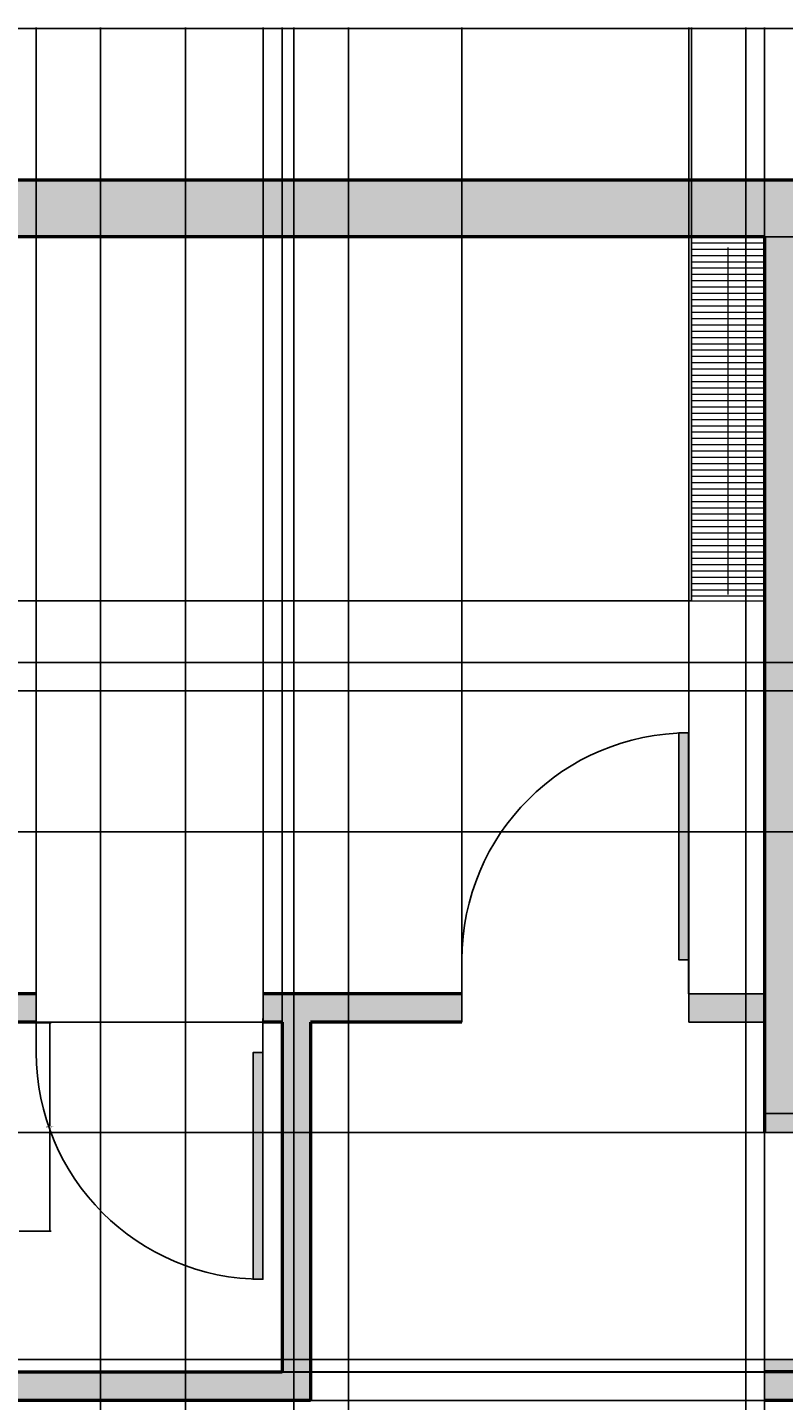
# Model space of a CAD drawing. Units: inches. Extents: x 1201 to 1754, y 247 to 775.
# Tile 8 of 10: x 1355 to 1475, y 557 to 775. Entities that reach past the tile are written whole.
import ezdxf

# ---------------------------------------------------------------- set-up
doc = ezdxf.new("R2010")
doc.units = ezdxf.units.IN
for name, color, linetype, lineweight in [('A-ANNO-DIMS', 2, 'Continuous', 18), ('A-DOOR', 4, 'Continuous', 25), ('A-FLOR-PANL', 8, 'Continuous', 18), ('A-FLOR-PANL-PATT', 8, 'Continuous', 13), ('A-WALL', 7, 'Continuous', 50), ('A-WALL-PATT', 9, 'Continuous', 13)]:
    doc.layers.add(name, color=color, linetype=linetype, lineweight=lineweight)
doc.layers.add('A-DOOR-PATT', color=29, linetype='Continuous', lineweight=13, true_color=0x4f342a)
doc.styles.get("Standard").update_dxf_attribs({"font": 'arial.ttf'})
doc.dimstyles.get("Standard").update_dxf_attribs({"dimtxt": 0.18, "dimasz": 0.18, "dimexe": 0.18, "dimexo": 0.0625, "dimgap": 0.09, "dimtad": 0, "dimtih": 1, "dimtoh": 1, "dimdec": 4, "dimzin": 0, "dimdsep": 46, "dimtxsty": 'Standard', "dimcen": 0.09, "dimadec": 0, "dimazin": 0, "dimtfac": 1, "dimtdec": 4, "dimtofl": 0, "dimtmove": 0, "dimatfit": 3, "dimfxl": 1, "dimtolj": 1, "dimtzin": 0, "dimarcsym": 0})

# ---------------------------------------------------------------- blocks, each defined once
blk = doc.blocks.new('*U2')
for p, q in [((0, 0), (0, -6)), ((-40, 0), (-40, -6))]:
    blk.add_line(p, q)
blk.add_lwpolyline([(0, 0), (0, 40), (-1.75, 40), (-1.75, 0)], close=True)
blk.add_arc((0, 0), 40, 90, 180)
blk = doc.blocks.new('*U3')
for p, q in [((0, 0), (0, -6)), ((40, 0), (40, -6))]:
    blk.add_line(p, q)
blk.add_lwpolyline([(0, 0), (0, 40), (1.75, 40), (1.75, 0)], close=True)
blk.add_arc((0, 0), 40, 0, 90)
blk = doc.blocks.new('*D27')
at = {"layer": 'A-ANNO-DIMS', "color": 0, "lineweight": -2, "transparency": 16777216}
for p, q in [((1353.29, 617.33), (1358.37, 617.33)), ((1358.19, 617.15), (1358.19, 600.99)), ((1358.19, 584.47), (1358.19, 600.63)), ((1353.29, 584.29), (1358.37, 584.29))]:
    blk.add_line(p, q, dxfattribs=at)
at = {"layer": 'A-ANNO-DIMS', "color": 0, "transparency": 16777216}
for points in [[(1358.16, 617.15), (1358.22, 617.15), (1358.19, 617.33)], [(1358.16, 584.47), (1358.22, 584.47), (1358.19, 584.29)]]:
    blk.add_solid(points, dxfattribs=at)
at = {"layer": 'Defpoints', "color": 0, "transparency": 16777216}
for p in [(1353.23, 617.33), (1358.19, 617.33), (1353.23, 584.29)]:
    blk.add_point(p, dxfattribs=at)
at = {"layer": 'A-ANNO-DIMS', "color": 0, "transparency": 16777216, "insert": (1358.19, 600.81), "char_height": 0.18, "attachment_point": 5}
blk.add_mtext('\\A1;WC 33 TYP.', dxfattribs=at)
blk = doc.blocks.new('*D45')
at = {"layer": 'A-ANNO-DIMS', "color": 0, "lineweight": -2, "transparency": 16777216}
for p, q in [((1246.52, 751), (1246.52, 775.14)), ((1726.52, 751), (1726.52, 775.14)), ((1246.7, 774.96), (1486.23, 774.96)), ((1726.34, 774.96), (1486.81, 774.96))]:
    blk.add_line(p, q, dxfattribs=at)
at = {"layer": 'A-ANNO-DIMS', "color": 0, "transparency": 16777216}
for points in [[(1246.7, 774.99), (1246.7, 774.93), (1246.52, 774.96)], [(1726.34, 774.99), (1726.34, 774.93), (1726.52, 774.96)]]:
    blk.add_solid(points, dxfattribs=at)
at = {"layer": 'Defpoints', "color": 0, "transparency": 16777216}
for p in [(1726.52, 774.96), (1246.52, 750.94), (1726.52, 750.94)]:
    blk.add_point(p, dxfattribs=at)
at = {"layer": 'A-ANNO-DIMS', "color": 0, "transparency": 16777216, "insert": (1486.52, 774.96), "char_height": 0.18, "attachment_point": 5}
blk.add_mtext('\\A1;480', dxfattribs=at)
blk = doc.blocks.new('*D47')
at = {"layer": 'A-ANNO-DIMS', "color": 0, "lineweight": -2, "transparency": 16777216}
for p, q in [((1255.52, 742), (1255.52, 775.14)), ((1471.52, 742), (1471.52, 775.14)), ((1255.7, 774.96), (1363.23, 774.96)), ((1471.34, 774.96), (1363.81, 774.96))]:
    blk.add_line(p, q, dxfattribs=at)
at = {"layer": 'A-ANNO-DIMS', "color": 0, "transparency": 16777216}
for points in [[(1255.7, 774.99), (1255.7, 774.93), (1255.52, 774.96)], [(1471.34, 774.99), (1471.34, 774.93), (1471.52, 774.96)]]:
    blk.add_solid(points, dxfattribs=at)
at = {"layer": 'Defpoints', "color": 0, "transparency": 16777216}
for p in [(1471.52, 774.96), (1255.52, 741.94), (1471.52, 741.94)]:
    blk.add_point(p, dxfattribs=at)
at = {"layer": 'A-ANNO-DIMS', "color": 0, "transparency": 16777216, "insert": (1363.52, 774.96), "char_height": 0.18, "attachment_point": 5}
blk.add_mtext('\\A1;216', dxfattribs=at)
blk = doc.blocks.new('*D49')
at = {"layer": 'A-ANNO-DIMS', "color": 0, "lineweight": -2, "transparency": 16777216}
for p, q in [((1394.96, 617.44), (1222.33, 617.44)), ((1222.51, 617.26), (1222.51, 589.87)), ((1222.51, 562.12), (1222.51, 589.51)), ((1394.96, 561.94), (1222.33, 561.94))]:
    blk.add_line(p, q, dxfattribs=at)
at = {"layer": 'A-ANNO-DIMS', "color": 0, "transparency": 16777216}
for points in [[(1222.48, 617.26), (1222.54, 617.26), (1222.51, 617.44)], [(1222.48, 562.12), (1222.54, 562.12), (1222.51, 561.94)]]:
    blk.add_solid(points, dxfattribs=at)
at = {"layer": 'Defpoints', "color": 0, "transparency": 16777216}
for p in [(1222.51, 617.44), (1395.02, 617.44), (1395.02, 561.94)]:
    blk.add_point(p, dxfattribs=at)
at = {"layer": 'A-ANNO-DIMS', "color": 0, "transparency": 16777216, "insert": (1222.51, 589.69), "char_height": 0.18, "attachment_point": 5}
blk.add_mtext('\\A1;55.5', dxfattribs=at)
blk = doc.blocks.new('*D52')
at = {"layer": 'A-ANNO-DIMS', "color": 0, "lineweight": -2, "transparency": 16777216}
for p, q in [((1477.46, 669.94), (1222.33, 669.94)), ((1222.51, 669.76), (1222.51, 616.12)), ((1222.51, 562.12), (1222.51, 615.76)), ((1477.46, 561.94), (1222.33, 561.94))]:
    blk.add_line(p, q, dxfattribs=at)
at = {"layer": 'A-ANNO-DIMS', "color": 0, "transparency": 16777216}
for points in [[(1222.48, 669.76), (1222.54, 669.76), (1222.51, 669.94)], [(1222.48, 562.12), (1222.54, 562.12), (1222.51, 561.94)]]:
    blk.add_solid(points, dxfattribs=at)
at = {"layer": 'Defpoints', "color": 0, "transparency": 16777216}
for p in [(1222.51, 669.94), (1477.52, 669.94), (1477.52, 561.94)]:
    blk.add_point(p, dxfattribs=at)
at = {"layer": 'A-ANNO-DIMS', "color": 0, "transparency": 16777216, "insert": (1222.51, 615.94), "char_height": 0.18, "attachment_point": 5}
blk.add_mtext('\\A1;108', dxfattribs=at)
blk = doc.blocks.new('*D53')
at = {"layer": 'A-ANNO-DIMS', "color": 0, "lineweight": -2, "transparency": 16777216}
for p, q in [((1717.46, 741.94), (1222.33, 741.94)), ((1222.51, 741.76), (1222.51, 708.37)), ((1222.51, 674.62), (1222.51, 708.01)), ((1657.46, 674.44), (1222.33, 674.44))]:
    blk.add_line(p, q, dxfattribs=at)
at = {"layer": 'A-ANNO-DIMS', "color": 0, "transparency": 16777216}
for points in [[(1222.48, 741.76), (1222.54, 741.76), (1222.51, 741.94)], [(1222.48, 674.62), (1222.54, 674.62), (1222.51, 674.44)]]:
    blk.add_solid(points, dxfattribs=at)
at = {"layer": 'Defpoints', "color": 0, "transparency": 16777216}
for p in [(1222.51, 741.94), (1717.52, 741.94), (1657.52, 674.44)]:
    blk.add_point(p, dxfattribs=at)
at = {"layer": 'A-ANNO-DIMS', "color": 0, "transparency": 16777216, "insert": (1222.51, 708.19), "char_height": 0.18, "attachment_point": 5}
blk.add_mtext('\\A1;67.5', dxfattribs=at)
blk = doc.blocks.new('*D54')
at = {"layer": 'A-ANNO-DIMS', "color": 0, "lineweight": -2, "transparency": 16777216}
for p, q in [((1255.52, 562), (1255.52, 775.14)), ((1395.02, 562), (1395.02, 775.14)), ((1255.7, 774.96), (1324.88, 774.96)), ((1394.84, 774.96), (1325.66, 774.96))]:
    blk.add_line(p, q, dxfattribs=at)
at = {"layer": 'A-ANNO-DIMS', "color": 0, "transparency": 16777216}
for points in [[(1255.7, 774.99), (1255.7, 774.93), (1255.52, 774.96)], [(1394.84, 774.99), (1394.84, 774.93), (1395.02, 774.96)]]:
    blk.add_solid(points, dxfattribs=at)
at = {"layer": 'Defpoints', "color": 0, "transparency": 16777216}
for p in [(1395.02, 774.96), (1255.52, 561.94), (1395.02, 561.94)]:
    blk.add_point(p, dxfattribs=at)
at = {"layer": 'A-ANNO-DIMS', "color": 0, "transparency": 16777216, "insert": (1325.27, 774.96), "char_height": 0.18, "attachment_point": 5}
blk.add_mtext('\\A1;139.5', dxfattribs=at)
blk = doc.blocks.new('*D58')
at = {"layer": 'A-ANNO-DIMS', "color": 0, "lineweight": -2, "transparency": 16777216}
for p, q in [((1405.52, 418), (1405.52, 775.14)), ((1468.52, 418), (1468.52, 775.14)), ((1405.7, 774.96), (1436.8, 774.96)), ((1468.34, 774.96), (1437.24, 774.96))]:
    blk.add_line(p, q, dxfattribs=at)
at = {"layer": 'A-ANNO-DIMS', "color": 0, "transparency": 16777216}
for points in [[(1405.7, 774.99), (1405.7, 774.93), (1405.52, 774.96)], [(1468.34, 774.99), (1468.34, 774.93), (1468.52, 774.96)]]:
    blk.add_solid(points, dxfattribs=at)
at = {"layer": 'Defpoints', "color": 0, "transparency": 16777216}
for p in [(1468.52, 774.96), (1405.52, 417.94), (1468.52, 417.94)]:
    blk.add_point(p, dxfattribs=at)
at = {"layer": 'A-ANNO-DIMS', "color": 0, "transparency": 16777216, "insert": (1437.02, 774.96), "char_height": 0.18, "attachment_point": 5}
blk.add_mtext('\\A1;63', dxfattribs=at)
blk = doc.blocks.new('*D59')
at = {"layer": 'A-ANNO-DIMS', "color": 0, "lineweight": -2, "transparency": 16777216}
for p, q in [((1255.52, 418), (1255.52, 775.14)), ((1405.52, 418), (1405.52, 775.14)), ((1255.7, 774.96), (1330.24, 774.96)), ((1405.34, 774.96), (1330.8, 774.96))]:
    blk.add_line(p, q, dxfattribs=at)
at = {"layer": 'A-ANNO-DIMS', "color": 0, "transparency": 16777216}
for points in [[(1255.7, 774.99), (1255.7, 774.93), (1255.52, 774.96)], [(1405.34, 774.99), (1405.34, 774.93), (1405.52, 774.96)]]:
    blk.add_solid(points, dxfattribs=at)
at = {"layer": 'Defpoints', "color": 0, "transparency": 16777216}
for p in [(1405.52, 774.96), (1255.52, 417.94), (1405.52, 417.94)]:
    blk.add_point(p, dxfattribs=at)
at = {"layer": 'A-ANNO-DIMS', "color": 0, "transparency": 16777216, "insert": (1330.52, 774.96), "char_height": 0.18, "attachment_point": 5}
blk.add_mtext('\\A1;150', dxfattribs=at)
blk = doc.blocks.new('*D61')
at = {"layer": 'A-ANNO-DIMS', "color": 0, "lineweight": -2, "transparency": 16777216}
for p, q in [((1423.52, 622), (1423.52, 775.14)), ((1459.52, 622), (1459.52, 775.14)), ((1423.7, 774.96), (1441.3, 774.96)), ((1459.34, 774.96), (1441.74, 774.96))]:
    blk.add_line(p, q, dxfattribs=at)
at = {"layer": 'A-ANNO-DIMS', "color": 0, "transparency": 16777216}
for points in [[(1423.7, 774.99), (1423.7, 774.93), (1423.52, 774.96)], [(1459.34, 774.99), (1459.34, 774.93), (1459.52, 774.96)]]:
    blk.add_solid(points, dxfattribs=at)
at = {"layer": 'Defpoints', "color": 0, "transparency": 16777216}
for p in [(1459.52, 774.96), (1423.52, 621.94), (1459.52, 621.94)]:
    blk.add_point(p, dxfattribs=at)
at = {"layer": 'A-ANNO-DIMS', "color": 0, "transparency": 16777216, "insert": (1441.52, 774.96), "char_height": 0.18, "attachment_point": 5}
blk.add_mtext('\\A1;36', dxfattribs=at)
blk = doc.blocks.new('*D62')
at = {"layer": 'A-ANNO-DIMS', "color": 0, "lineweight": -2, "transparency": 16777216}
for p, q in [((1459.52, 622), (1459.52, 775.14)), ((1471.52, 622), (1471.52, 775.14)), ((1459.7, 774.96), (1465.31, 774.96)), ((1471.34, 774.96), (1465.73, 774.96))]:
    blk.add_line(p, q, dxfattribs=at)
at = {"layer": 'A-ANNO-DIMS', "color": 0, "transparency": 16777216}
for points in [[(1459.7, 774.99), (1459.7, 774.93), (1459.52, 774.96)], [(1471.34, 774.99), (1471.34, 774.93), (1471.52, 774.96)]]:
    blk.add_solid(points, dxfattribs=at)
at = {"layer": 'Defpoints', "color": 0, "transparency": 16777216}
for p in [(1471.52, 774.96), (1459.52, 621.94), (1471.52, 621.94)]:
    blk.add_point(p, dxfattribs=at)
at = {"layer": 'A-ANNO-DIMS', "color": 0, "transparency": 16777216, "insert": (1465.52, 774.96), "char_height": 0.18, "attachment_point": 5}
blk.add_mtext('\\A1;12', dxfattribs=at)
blk = doc.blocks.new('*D63')
at = {"layer": 'A-ANNO-DIMS', "color": 0, "lineweight": -2, "transparency": 16777216}
for p, q in [((1356.02, 622), (1356.02, 775.14)), ((1392.02, 622), (1392.02, 775.14)), ((1356.2, 774.96), (1373.8, 774.96)), ((1391.84, 774.96), (1374.24, 774.96))]:
    blk.add_line(p, q, dxfattribs=at)
at = {"layer": 'A-ANNO-DIMS', "color": 0, "transparency": 16777216}
for points in [[(1356.2, 774.99), (1356.2, 774.93), (1356.02, 774.96)], [(1391.84, 774.99), (1391.84, 774.93), (1392.02, 774.96)]]:
    blk.add_solid(points, dxfattribs=at)
at = {"layer": 'Defpoints', "color": 0, "transparency": 16777216}
for p in [(1392.02, 774.96), (1356.02, 621.94), (1392.02, 621.94)]:
    blk.add_point(p, dxfattribs=at)
at = {"layer": 'A-ANNO-DIMS', "color": 0, "transparency": 16777216, "insert": (1374.02, 774.96), "char_height": 0.18, "attachment_point": 5}
blk.add_mtext('\\A1;36', dxfattribs=at)
blk = doc.blocks.new('*D64')
at = {"layer": 'A-ANNO-DIMS', "color": 0, "lineweight": -2, "transparency": 16777216}
for p, q in [((1392.02, 622), (1392.02, 775.14)), ((1423.52, 622), (1423.52, 775.14)), ((1392.2, 774.96), (1407.45, 774.96)), ((1423.34, 774.96), (1408.1, 774.96))]:
    blk.add_line(p, q, dxfattribs=at)
at = {"layer": 'A-ANNO-DIMS', "color": 0, "transparency": 16777216}
for points in [[(1392.2, 774.99), (1392.2, 774.93), (1392.02, 774.96)], [(1423.34, 774.99), (1423.34, 774.93), (1423.52, 774.96)]]:
    blk.add_solid(points, dxfattribs=at)
at = {"layer": 'Defpoints', "color": 0, "transparency": 16777216}
for p in [(1423.52, 774.96), (1392.02, 621.94), (1423.52, 621.94)]:
    blk.add_point(p, dxfattribs=at)
at = {"layer": 'A-ANNO-DIMS', "color": 0, "transparency": 16777216, "insert": (1407.77, 774.96), "char_height": 0.18, "attachment_point": 5}
blk.add_mtext('\\A1;31.5', dxfattribs=at)
blk = doc.blocks.new('*D65')
at = {"layer": 'A-ANNO-DIMS', "color": 0, "lineweight": -2, "transparency": 16777216}
for p, q in [((1471.46, 599.94), (1222.33, 599.94)), ((1222.51, 599.76), (1222.51, 582.12)), ((1222.51, 564.12), (1222.51, 581.76)), ((1471.46, 563.94), (1222.33, 563.94))]:
    blk.add_line(p, q, dxfattribs=at)
at = {"layer": 'A-ANNO-DIMS', "color": 0, "transparency": 16777216}
for points in [[(1222.48, 599.76), (1222.54, 599.76), (1222.51, 599.94)], [(1222.48, 564.12), (1222.54, 564.12), (1222.51, 563.94)]]:
    blk.add_solid(points, dxfattribs=at)
at = {"layer": 'Defpoints', "color": 0, "transparency": 16777216}
for p in [(1222.51, 599.94), (1471.52, 599.94), (1471.52, 563.94)]:
    blk.add_point(p, dxfattribs=at)
at = {"layer": 'A-ANNO-DIMS', "color": 0, "transparency": 16777216, "insert": (1222.51, 581.94), "char_height": 0.18, "attachment_point": 5}
blk.add_mtext('\\A1;36', dxfattribs=at)
blk = doc.blocks.new('*D76')
at = {"layer": 'A-ANNO-DIMS', "color": 0, "lineweight": -2, "transparency": 16777216}
for p, q in [((1717.46, 669.94), (1222.33, 669.94)), ((1222.51, 669.76), (1222.51, 658.95)), ((1222.51, 647.78), (1222.51, 658.59)), ((1717.46, 647.6), (1222.33, 647.6))]:
    blk.add_line(p, q, dxfattribs=at)
at = {"layer": 'A-ANNO-DIMS', "color": 0, "transparency": 16777216}
for points in [[(1222.48, 669.76), (1222.54, 669.76), (1222.51, 669.94)], [(1222.48, 647.78), (1222.54, 647.78), (1222.51, 647.6)]]:
    blk.add_solid(points, dxfattribs=at)
at = {"layer": 'Defpoints', "color": 0, "transparency": 16777216}
for p in [(1222.51, 669.94), (1717.52, 669.94), (1717.52, 647.6)]:
    blk.add_point(p, dxfattribs=at)
at = {"layer": 'A-ANNO-DIMS', "color": 0, "transparency": 16777216, "insert": (1222.51, 658.77), "char_height": 0.18, "attachment_point": 5}
blk.add_mtext('\\A1;22.34', dxfattribs=at)
blk = doc.blocks.new('*D83')
at = {"layer": 'A-ANNO-DIMS', "color": 0, "lineweight": -2, "transparency": 16777216}
for p, q in [((1471.46, 561.97), (1222.33, 561.97)), ((1222.51, 561.79), (1222.51, 559.89)), ((1222.51, 557.62), (1222.51, 559.52)), ((1471.46, 557.44), (1222.33, 557.44))]:
    blk.add_line(p, q, dxfattribs=at)
at = {"layer": 'A-ANNO-DIMS', "color": 0, "transparency": 16777216}
for points in [[(1222.48, 561.79), (1222.54, 561.79), (1222.51, 561.97)], [(1222.48, 557.62), (1222.54, 557.62), (1222.51, 557.44)]]:
    blk.add_solid(points, dxfattribs=at)
at = {"layer": 'Defpoints', "color": 0, "transparency": 16777216}
for p in [(1222.51, 561.97), (1471.52, 561.97), (1471.52, 557.44)]:
    blk.add_point(p, dxfattribs=at)
at = {"layer": 'A-ANNO-DIMS', "color": 0, "transparency": 16777216, "insert": (1222.51, 559.71), "char_height": 0.18, "attachment_point": 5}
blk.add_mtext('\\A1;4.528', dxfattribs=at)
blk = doc.blocks.new('*D84')
at = {"layer": 'A-ANNO-DIMS', "color": 0, "lineweight": -2, "transparency": 16777216}
for p, q in [((1471.52, 600), (1471.52, 775.14)), ((1477.52, 600), (1477.52, 775.14)), ((1471.7, 774.96), (1474.37, 774.96)), ((1477.34, 774.96), (1474.67, 774.96))]:
    blk.add_line(p, q, dxfattribs=at)
at = {"layer": 'A-ANNO-DIMS', "color": 0, "transparency": 16777216}
for points in [[(1471.7, 774.99), (1471.7, 774.93), (1471.52, 774.96)], [(1477.34, 774.99), (1477.34, 774.93), (1477.52, 774.96)]]:
    blk.add_solid(points, dxfattribs=at)
at = {"layer": 'Defpoints', "color": 0, "transparency": 16777216}
for p in [(1477.52, 774.96), (1471.52, 599.94), (1477.52, 599.94)]:
    blk.add_point(p, dxfattribs=at)
at = {"layer": 'A-ANNO-DIMS', "color": 0, "transparency": 16777216, "insert": (1474.52, 774.96), "char_height": 0.18, "attachment_point": 5}
blk.add_mtext('\\A1;6', dxfattribs=at)
blk = doc.blocks.new('*D87')
at = {"layer": 'A-ANNO-DIMS', "color": 0, "lineweight": -2, "transparency": 16777216}
for p, q in [((1459.84, 741.94), (1222.33, 741.94)), ((1222.51, 741.76), (1222.51, 713.27)), ((1222.51, 684.41), (1222.51, 712.91)), ((1459.84, 684.23), (1222.33, 684.23))]:
    blk.add_line(p, q, dxfattribs=at)
at = {"layer": 'A-ANNO-DIMS', "color": 0, "transparency": 16777216}
for points in [[(1222.48, 741.76), (1222.54, 741.76), (1222.51, 741.94)], [(1222.48, 684.41), (1222.54, 684.41), (1222.51, 684.23)]]:
    blk.add_solid(points, dxfattribs=at)
at = {"layer": 'Defpoints', "color": 0, "transparency": 16777216}
for p in [(1222.51, 741.94), (1459.9, 741.94), (1459.9, 684.23)]:
    blk.add_point(p, dxfattribs=at)
at = {"layer": 'A-ANNO-DIMS', "color": 0, "transparency": 16777216, "insert": (1222.51, 713.09), "char_height": 0.18, "attachment_point": 5}
blk.add_mtext('\\A1;57.71', dxfattribs=at)
blk = doc.blocks.new('*D88')
at = {"layer": 'A-ANNO-DIMS', "color": 0, "lineweight": -2, "transparency": 16777216}
for p, q in [((1459.9, 684.3), (1459.9, 775.14)), ((1471.52, 684.3), (1471.52, 775.14)), ((1460.08, 774.96), (1465.25, 774.96)), ((1471.34, 774.96), (1466.16, 774.96))]:
    blk.add_line(p, q, dxfattribs=at)
at = {"layer": 'A-ANNO-DIMS', "color": 0, "transparency": 16777216}
for points in [[(1460.08, 774.99), (1460.08, 774.93), (1459.9, 774.96)], [(1471.34, 774.99), (1471.34, 774.93), (1471.52, 774.96)]]:
    blk.add_solid(points, dxfattribs=at)
at = {"layer": 'Defpoints', "color": 0, "transparency": 16777216}
for p in [(1471.52, 774.96), (1459.9, 684.23), (1471.52, 684.23)]:
    blk.add_point(p, dxfattribs=at)
at = {"layer": 'A-ANNO-DIMS', "color": 0, "transparency": 16777216, "insert": (1465.71, 774.96), "char_height": 0.18, "attachment_point": 5}
blk.add_mtext('\\A1;11.623', dxfattribs=at)
blk = doc.blocks.new('*D89')
at = {"layer": 'A-ANNO-DIMS', "color": 0, "lineweight": -2, "transparency": 16777216}
for p, q in [((1396.89, 281.58), (1396.89, 775.14)), ((1471.52, 280), (1471.52, 775.14)), ((1397.07, 774.96), (1433.81, 774.96)), ((1471.34, 774.96), (1434.6, 774.96))]:
    blk.add_line(p, q, dxfattribs=at)
at = {"layer": 'A-ANNO-DIMS', "color": 0, "transparency": 16777216}
for points in [[(1397.07, 774.99), (1397.07, 774.93), (1396.89, 774.96)], [(1471.34, 774.99), (1471.34, 774.93), (1471.52, 774.96)]]:
    blk.add_solid(points, dxfattribs=at)
at = {"layer": 'Defpoints', "color": 0, "transparency": 16777216}
for p in [(1471.52, 774.96), (1396.89, 281.52), (1471.52, 279.94)]:
    blk.add_point(p, dxfattribs=at)
at = {"layer": 'A-ANNO-DIMS', "color": 0, "transparency": 16777216, "insert": (1434.21, 774.96), "char_height": 0.18, "attachment_point": 5}
blk.add_mtext('\\A1;74.63', dxfattribs=at)
blk = doc.blocks.new('*D98')
at = {"layer": 'A-ANNO-DIMS', "color": 0, "lineweight": -2, "transparency": 16777216}
for p, q in [((1366.21, 509.65), (1366.21, 775.14)), ((1379.71, 519.97), (1379.71, 775.14)), ((1366.39, 774.96), (1372.5, 774.96)), ((1379.53, 774.96), (1373.41, 774.96))]:
    blk.add_line(p, q, dxfattribs=at)
at = {"layer": 'A-ANNO-DIMS', "color": 0, "transparency": 16777216}
for points in [[(1366.39, 774.99), (1366.39, 774.93), (1366.21, 774.96)], [(1379.53, 774.99), (1379.53, 774.93), (1379.71, 774.96)]]:
    blk.add_solid(points, dxfattribs=at)
at = {"layer": 'Defpoints', "color": 0, "transparency": 16777216}
for p in [(1379.71, 774.96), (1379.71, 519.9), (1366.21, 509.58)]:
    blk.add_point(p, dxfattribs=at)
at = {"layer": 'A-ANNO-DIMS', "color": 0, "transparency": 16777216, "insert": (1372.96, 774.96), "char_height": 0.18, "attachment_point": 5}
blk.add_mtext('\\A1;13.494', dxfattribs=at)

msp = doc.modelspace()

# ---------------------------------------------------------------- hatches: boundary and pattern name
at = {"layer": 'A-DOOR-PATT'}
h = msp.add_hatch(color=256, dxfattribs=at)
h.dxf.hatch_style = 1
h.paths.add_polyline_path([(1391.9756, 612.6194), (1390.4026, 612.6194), (1390.4026, 576.699, 0.01094143), (1391.9756, 576.6646)])
h.paths.add_polyline_path([(1471.5208, 621.9415), (1459.5208, 621.9415), (1459.5208, 617.4415), (1471.5208, 617.4415)])
h.paths.add_polyline_path([(1459.4756, 663.2896, 0.01094143), (1457.9026, 663.2551), (1457.9026, 627.3347), (1459.4756, 627.3347)])
h.paths.add_polyline_path([(1477.5208, 602.9415), (1471.5208, 602.9415), (1471.5208, 599.9415), (1477.5208, 599.9415)])
h.paths.add_polyline_path([(1518.8344, 565.5145), (1482.914, 565.5145), (1482.914, 563.9415), (1518.8689, 563.9415, 0.01094143)])
h.paths.add_polyline_path([(1477.5208, 563.9415), (1471.5208, 563.9415), (1471.5208, 561.9692), (1477.5208, 561.9692)])
h.paths.add_polyline_path([(1621.5208, 674.4415), (1618.5208, 674.4415), (1618.5208, 669.9415), (1621.5208, 669.9415)])
h.paths.add_polyline_path([(1660.5208, 674.4415), (1657.5208, 674.4415), (1657.5208, 669.9415), (1660.5208, 669.9415)])
h.paths.add_polyline_path([(1657.509, 715.7896, 0.01094143), (1655.936, 715.7551), (1655.936, 679.8347), (1657.509, 679.8347)])
h.paths.add_polyline_path([(1566.0208, 279.9415), (1563.0208, 279.9415), (1563.0208, 270.9415), (1566.0208, 270.9415)])
h.paths.add_polyline_path([(1567.6389, 321.2551, 0.01094143), (1566.0659, 321.2896), (1566.0659, 285.3347), (1567.6389, 285.3347)])
h.paths.add_polyline_path([(1603.0208, 279.9415), (1602.0208, 279.9415), (1602.0208, 270.9415), (1603.0208, 270.9415)])
h.paths.add_polyline_path([(1641.0208, 279.9415), (1638.0208, 279.9415), (1638.0208, 270.9415), (1641.0208, 270.9415)])
h.paths.add_polyline_path([(1638.0208, 320.3922, 0.01094143), (1636.4477, 320.3578), (1636.4477, 284.4374), (1638.0208, 284.4374)])
at = {"layer": 'A-FLOR-PANL-PATT'}
h = msp.add_hatch(dxfattribs=at)
h.set_pattern_fill('ANSI31', color=256, scale=0.3149606, angle=-45, style=0)
h.paths.add_polyline_path([(1459.8979, 684.2327), (1471.5208, 684.2327), (1471.5208, 741.9415), (1459.8979, 741.9415)])
at = {"layer": 'A-WALL-PATT'}
h = msp.add_hatch(color=256, dxfattribs=at)
h.dxf.hatch_style = 1
h.paths.add_polyline_path([(1255.5208, 741.9415), (1471.5208, 741.9415), (1471.5208, 684.2327), (1471.5208, 602.9415), (1477.5208, 602.9415), (1477.5208, 669.9415), (1618.5208, 669.9415), (1618.5208, 674.4415), (1477.5208, 674.4415), (1477.5208, 741.9415), (1481.2969, 741.9415), (1481.2969, 750.9415), (1246.5208, 750.9415), (1246.5208, 700.7954), (1255.5208, 700.7954)])
h.paths.add_polyline_path([(1255.5208, 557.4415), (1399.5208, 557.4415), (1399.5208, 617.4415), (1423.5208, 617.4415), (1423.5208, 621.9415), (1392.0208, 621.9415), (1392.0208, 617.4415), (1395.0208, 617.4415), (1395.0208, 561.9415), (1255.5208, 561.9415), (1255.5208, 571.8878), (1246.5208, 571.8878), (1246.5208, 506.6967), (1255.5208, 506.6967)])
h.paths.add_polyline_path([(1255.5208, 664.7954), (1246.5208, 664.7954), (1246.5208, 595.8878), (1255.398, 595.8878), (1255.398, 617.4415), (1315.398, 617.4415), (1356.0208, 617.4415), (1356.0208, 618.0127), (1356.0208, 621.9415), (1255.5208, 621.9415), (1255.5208, 629.6628)])
h.paths.add_polyline_path([(1255.5208, 470.6967), (1246.5208, 470.6967), (1246.5208, 347.7487), (1255.5208, 347.7487), (1255.5208, 413.4415), (1405.5208, 413.4415), (1405.5208, 417.9415), (1255.5208, 417.9415)])
h.paths.add_polyline_path([(1290.9481, 279.9415), (1255.5208, 279.9415), (1255.5208, 311.7487), (1246.5208, 311.7487), (1246.5208, 270.9415), (1290.9481, 270.9415)])
h.paths.add_polyline_path([(1486.5907, 279.9415), (1477.5208, 279.9415), (1477.5208, 417.9415), (1468.5208, 417.9415), (1468.5208, 413.4415), (1471.5208, 413.4415), (1471.5208, 279.9415), (1399.0105, 279.9415), (1399.0105, 270.9415), (1486.5907, 270.9415)])
h.paths.add_polyline_path([(1563.0208, 279.9415), (1542.0208, 279.9415), (1542.0208, 417.9415), (1501.5208, 417.9415), (1501.5208, 413.4415), (1513.81, 413.4415), (1513.8125, 413.6987), (1537.8114, 413.4623), (1537.5208, 383.9637), (1537.5208, 279.9415), (1522.5907, 279.9415), (1522.5907, 270.9415), (1563.0208, 270.9415)])
h.paths.add_polyline_path([(1726.5208, 404.0342), (1717.5208, 404.0342), (1717.5208, 279.9415), (1641.0208, 279.9415), (1641.0208, 270.9415), (1726.5208, 270.9415)])
h.paths.add_polyline_path([(1726.5208, 507.4363), (1717.5208, 507.4363), (1717.5208, 440.0342), (1726.5208, 440.0342)])
h.paths.add_polyline_path([(1726.5208, 611.6009), (1717.5208, 611.6009), (1717.5208, 561.9415), (1477.5208, 561.9415), (1471.5208, 561.9692), (1471.5208, 557.4415), (1717.5208, 557.4415), (1717.5208, 543.4363), (1726.5208, 543.4363)])
h.paths.add_polyline_path([(1726.5208, 750.9415), (1505.2969, 750.9415), (1505.2969, 741.9415), (1697.6884, 741.9415), (1697.6884, 741.9922), (1718.6884, 741.9922), (1718.6884, 733.9922), (1717.5208, 733.9922), (1717.5208, 674.4415), (1660.5208, 674.4415), (1660.5208, 669.9415), (1717.5208, 669.9415), (1717.5208, 647.6009), (1726.5208, 647.6009)])

# ---------------------------------------------------------------- linework, layer by layer
at = {"layer": 'A-DOOR'}
for p, q in [((1356.0208, 621.9415), (1356.0208, 612.6194)), ((1392.0208, 621.9415), (1392.0208, 617.4415)), ((1423.5208, 621.9415), (1423.5208, 617.4415)), ((1471.5208, 621.9415), (1459.5208, 621.9415)), ((1459.5208, 621.9415), (1459.5208, 617.4415)), ((1471.5208, 617.4415), (1459.5208, 617.4415)), ((1477.5208, 602.9415), (1471.5208, 602.9415)), ((1477.5208, 599.9415), (1471.5208, 599.9415)), ((1477.5208, 563.9415), (1471.5208, 563.9415)), ((1471.5208, 563.9415), (1471.5208, 557.4415))]:
    msp.add_line(p, q, dxfattribs=at)
at = {"layer": 'A-FLOR-PANL'}
for p, q in [((1471.5208, 741.9415), (1459.8979, 741.9415)), ((1459.8979, 741.9415), (1459.8979, 684.2327)), ((1465.7093, 740.2327), (1465.7093, 685.2327)), ((1471.5208, 684.2327), (1471.5208, 741.9415)), ((1459.8979, 684.2327), (1471.5208, 684.2327))]:
    msp.add_line(p, q, dxfattribs=at)
at = {"layer": 'A-WALL'}
for p, q in [((1471.5208, 741.9415), (1255.5208, 741.9415)), ((1471.5208, 741.9415), (1471.5208, 599.9415)), ((1356.0208, 621.9415), (1255.5208, 621.9415)), ((1423.5208, 621.9415), (1392.0208, 621.9415)), ((1356.0208, 617.4415), (1255.5208, 617.4415)), ((1395.0208, 617.4415), (1392.0208, 617.4415)), ((1395.0208, 617.4415), (1395.0208, 561.9415)), ((1399.5208, 617.4415), (1399.5208, 557.4415)), ((1399.5208, 617.4415), (1399.5208, 557.4415)), ((1423.5208, 617.4415), (1399.5208, 617.4415)), ((1395.0208, 561.9415), (1255.5208, 561.9415)), ((1395.0208, 561.9415), (1356.0208, 561.9415)), ((1674.7834, 561.9692), (1471.5208, 561.9692)), ((1399.5208, 557.4415), (1255.5208, 557.4415)), ((1717.5208, 557.4415), (1471.5208, 557.4415))]:
    msp.add_line(p, q, dxfattribs=at)
msp.add_lwpolyline([(1638.0208, 270.9415), (1726.5208, 270.9415), (1726.5208, 750.9415), (1246.5208, 750.9415), (1246.5208, 270.9415), (1566.0208, 270.9415)], dxfattribs=at)

# ---------------------------------------------------------------- block references
at = {"layer": 'A-DOOR', "xscale": 0.8988714898198789, "yscale": 0.8988714898198789, "zscale": 0.8988714898198789}
msp.add_blockref('*U2', (1459.4756, 627.3347), dxfattribs=at)
at = {"layer": 'A-DOOR', "xscale": 0.8988714898198789, "yscale": 0.8988714898198789, "zscale": 0.8988714898198789, "rotation": 180}
msp.add_blockref('*U3', (1391.9756, 612.6194), dxfattribs=at)

# ---------------------------------------------------------------- dimensions: what is measured, and where the dimension line sits
at = {"layer": 'A-ANNO-DIMS'}
for base, p1, p2, override, picture, middle in [((1726.5208, 774.9565), (1246.5208, 750.9415), (1726.5208, 750.9415), {"dimdec": 0, "dimlfac": 1, "dimrnd": 0, "dimzin": 0, "dimdsep": 46, "dimlunit": 2}, '*D45', (1486.5208, 774.9565)), ((1471.5208, 774.9565), (1255.5208, 741.9415), (1471.5208, 741.9415), {"dimdec": 0, "dimlfac": 1, "dimrnd": 0, "dimzin": 0, "dimdsep": 46, "dimlunit": 2}, '*D47', (1363.5208, 774.9565)), ((1395.0208, 774.9565), (1255.5208, 561.9415), (1395.0208, 561.9415), {"dimdec": 1, "dimlfac": 1, "dimrnd": 0, "dimzin": 0, "dimdsep": 46, "dimlunit": 2}, '*D54', (1325.2708, 774.9565)), ((1405.5208, 774.9565), (1255.5208, 417.9415), (1405.5208, 417.9415), {"dimdec": 0, "dimlfac": 1, "dimrnd": 0, "dimzin": 0, "dimdsep": 46, "dimlunit": 2}, '*D59', (1330.5208, 774.9565)), ((1392.0208, 774.9565), (1356.0208, 621.9415), (1392.0208, 621.9415), {"dimdec": 0, "dimlfac": 1, "dimrnd": 0, "dimzin": 0, "dimdsep": 46, "dimlunit": 2}, '*D63', (1374.0208, 774.9565)), ((1379.7057, 774.9565), (1366.2113, 509.5839), (1379.7057, 519.9035), {"dimdec": 3, "dimlfac": 1, "dimrnd": 0, "dimzin": 0, "dimdsep": 46, "dimlunit": 2}, '*D98', (1372.9585, 774.9565)), ((1423.5208, 774.9565), (1392.0208, 621.9415), (1423.5208, 621.9415), {"dimdec": 1, "dimlfac": 1, "dimrnd": 0, "dimzin": 0, "dimdsep": 46, "dimlunit": 2}, '*D64', (1407.7708, 774.9565)), ((1471.5208, 774.9565), (1396.8927, 281.5161), (1471.5208, 279.9415), {"dimdec": 2, "dimlfac": 1, "dimrnd": 0, "dimzin": 0, "dimdsep": 46, "dimlunit": 2}, '*D89', (1434.2067, 774.9565)), ((1468.5208, 774.9565), (1405.5208, 417.9415), (1468.5208, 417.9415), {"dimdec": 0, "dimlfac": 1, "dimrnd": 0, "dimzin": 0, "dimdsep": 46, "dimlunit": 2}, '*D58', (1437.0208, 774.9565)), ((1459.5208, 774.9565), (1423.5208, 621.9415), (1459.5208, 621.9415), {"dimdec": 0, "dimlfac": 1, "dimrnd": 0, "dimzin": 0, "dimdsep": 46, "dimlunit": 2}, '*D61', (1441.5208, 774.9565)), ((1471.5208, 774.9565), (1459.5208, 621.9415), (1471.5208, 621.9415), {"dimdec": 0, "dimlfac": 1, "dimrnd": 0, "dimzin": 0, "dimdsep": 46, "dimlunit": 2}, '*D62', (1465.5208, 774.9565)), ((1471.5208, 774.9565), (1459.8979, 684.2327), (1471.5208, 684.2327), {"dimdec": 3, "dimlfac": 1, "dimrnd": 0, "dimzin": 0, "dimdsep": 46, "dimlunit": 2}, '*D88', (1465.7093, 774.9565)), ((1477.5208, 774.9565), (1471.5208, 599.9415), (1477.5208, 599.9415), {"dimdec": 0, "dimlfac": 1, "dimrnd": 0, "dimzin": 0, "dimdsep": 46, "dimlunit": 2}, '*D84', (1474.5208, 774.9565))]:
    dim = msp.add_linear_dim(base=base, p1=p1, p2=p2, dimstyle='Standard', override=override, dxfattribs=at)
    dim.commit()
    dim.dimension.update_dxf_attribs({"geometry": picture, "text_midpoint": middle})
for base, p1, p2, override, picture, middle in [((1222.5058, 741.9415), (1459.8979, 684.2327), (1459.8979, 741.9415), {"dimdec": 2, "dimlfac": 1, "dimrnd": 0, "dimzin": 0, "dimdsep": 46, "dimlunit": 2}, '*D87', (1222.5058, 713.0871)), ((1222.5058, 741.9415), (1657.5208, 674.4415), (1717.5208, 741.9415), {"dimdec": 1, "dimlfac": 1, "dimrnd": 0, "dimzin": 0, "dimdsep": 46, "dimlunit": 2}, '*D53', (1222.5058, 708.1915)), ((1222.5058, 669.9415), (1717.5208, 647.6009), (1717.5208, 669.9415), {"dimdec": 2, "dimlfac": 1, "dimrnd": 0, "dimzin": 0, "dimdsep": 46, "dimlunit": 2}, '*D76', (1222.5058, 658.7712)), ((1222.5058, 669.9415), (1477.5208, 561.9415), (1477.5208, 669.9415), {"dimdec": 0, "dimlfac": 1, "dimrnd": 0, "dimzin": 0, "dimdsep": 46, "dimlunit": 2}, '*D52', (1222.5058, 615.9415)), ((1222.5058, 617.4415), (1395.0208, 561.9415), (1395.0208, 617.4415), {"dimdec": 1, "dimlfac": 1, "dimrnd": 0, "dimzin": 0, "dimdsep": 46, "dimlunit": 2}, '*D49', (1222.5058, 589.6915)), ((1222.5058, 599.9415), (1471.5208, 563.9415), (1471.5208, 599.9415), {"dimdec": 0, "dimlfac": 1, "dimrnd": 0, "dimzin": 0, "dimdsep": 46, "dimlunit": 2}, '*D65', (1222.5058, 581.9415)), ((1222.5058, 561.9692), (1471.5208, 557.4415), (1471.5208, 561.9692), {"dimdec": 3, "dimlfac": 1, "dimrnd": 0, "dimzin": 0, "dimdsep": 46, "dimlunit": 2}, '*D83', (1222.5058, 559.7053))]:
    dim = msp.add_linear_dim(base=base, p1=p1, p2=p2, angle=90, dimstyle='Standard', override=override, dxfattribs=at)
    dim.commit()
    dim.dimension.update_dxf_attribs({"geometry": picture, "text_midpoint": middle})
dim = msp.add_linear_dim(base=(1358.1885, 617.3316), p1=(1353.2316, 584.2854), p2=(1353.2316, 617.3316), angle=90, text='WC <> TYP.', dimstyle='Standard', override={"dimdec": 0, "dimlfac": 1, "dimrnd": 0, "dimzin": 0, "dimdsep": 46, "dimlunit": 2}, dxfattribs=at)
dim.commit()
dim.dimension.update_dxf_attribs({"geometry": '*D27', "text_midpoint": (1358.1885, 600.8085)})

doc.saveas('drawing.dxf')
